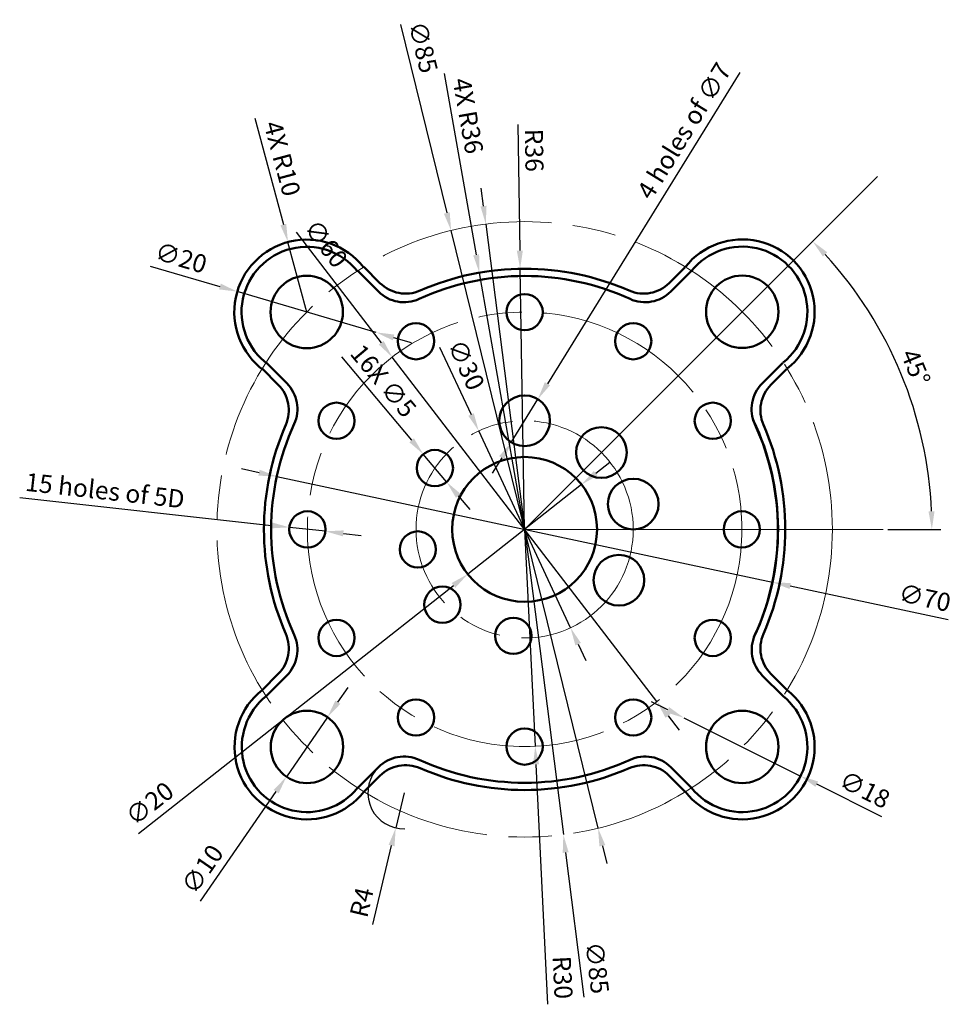
# Model space of a CAD drawing. Units: millimetres. Extents: x 2004 to 2133, y 1449 to 1585.
import ezdxf

# ---------------------------------------------------------------- set-up
doc = ezdxf.new("R2010")
doc.units = ezdxf.units.MM
doc.linetypes.add('ACAD_ISO08W100', pattern=[36, 24, -3, 6, -3])
for name, color, linetype, lineweight in [('M-CNTR', 4, 'ACAD_ISO08W100', 18), ('M-CONS', 8, 'Continuous', 18), ('M-DIMS', 2, 'Continuous', 25), ('M-OUTL', 7, 'Continuous', 50)]:
    doc.layers.add(name, color=color, linetype=linetype, lineweight=lineweight)
doc.styles.get("Standard").update_dxf_attribs({"font": 'arial.ttf'})
doc.dimstyles.new('ISO-25', dxfattribs={"dimtxt": 2.5, "dimasz": 2.5, "dimexe": 1.25, "dimexo": 0.625, "dimtad": 1, "dimdec": 1, "dimdsep": 46, "dimtxsty": 'Standard', "dimcen": 2.5, "dimadec": 0, "dimazin": 0, "dimtfac": 1, "dimtdec": 1, "dimtmove": 0, "dimatfit": 3, "dimfxl": 1, "dimarcsym": 0})

# ---------------------------------------------------------------- blocks, each defined once
blk = doc.blocks.new('*U1')
blk.add_circle((0, 0), 2.5)
blk = doc.blocks.new('*U2')
at = {"layer": 'M-OUTL', "color": 0, "linetype": 'ByBlock', "lineweight": -2, "transparency": 16777216}
blk.add_blockref('*U1', (2074.15, 1544.97), dxfattribs=at)
for p, rotation in [((2059.15, 1540.95), 30), ((2089.15, 1540.95), 330.0000000000001), ((2048.17, 1529.97), 59.99999999999999), ((2100.13, 1529.97), 300), ((2044.15, 1514.97), 90), ((2104.15, 1514.97), 269.9999999999999), ((2048.17, 1499.97), 120), ((2100.13, 1499.97), 240), ((2059.15, 1488.99), 150), ((2089.15, 1488.99), 210), ((2074.15, 1484.97), 180)]:
    blk.add_blockref('*U1', p, dxfattribs=dict(at, rotation=rotation))
blk = doc.blocks.new('*D3')
at = {"layer": 'Defpoints', "color": 0, "lineweight": 100, "transparency": 16777216}
for p in [(2073.53, 1550.97), (2074.15, 1514.97)]:
    blk.add_point(p, dxfattribs=at)
at = {"layer": 'M-DIMS', "color": 0, "lineweight": -2, "transparency": 16777216}
for p, q in [((2073.19, 1570.9), (2073.49, 1553.47)), ((2074.15, 1514.97), (2073.53, 1550.97))]:
    blk.add_line(p, q, dxfattribs=at)
at = {"layer": 'M-DIMS', "color": 0, "lineweight": 100, "transparency": 16777216}
blk.add_solid([(2073.91, 1553.47), (2073.07, 1553.46), (2073.53, 1550.97)], dxfattribs=at)
at = {"layer": 'M-DIMS', "color": 0, "transparency": 16777216, "insert": (2075.15, 1567.32), "char_height": 2.5, "attachment_point": 5, "rotation": 270.9785}
blk.add_mtext('R36', dxfattribs=at)
blk = doc.blocks.new('*D4')
at = {"layer": 'Defpoints', "color": 0, "lineweight": 100, "transparency": 16777216}
for p in [(2034.47, 1547.81), (2053.66, 1542.18)]:
    blk.add_point(p, dxfattribs=at)
at = {"layer": 'M-DIMS', "color": 0, "lineweight": -2, "transparency": 16777216}
for p, q in [((2022.43, 1551.34), (2032.07, 1548.51)), ((2053.66, 1542.18), (2034.47, 1547.81)), ((2056.06, 1541.47), (2058.46, 1540.77))]:
    blk.add_line(p, q, dxfattribs=at)
at = {"layer": 'M-DIMS', "color": 0, "lineweight": 100, "transparency": 16777216}
for points in [[(2032.19, 1548.91), (2031.95, 1548.11), (2034.47, 1547.81)], [(2056.17, 1541.87), (2055.94, 1541.07), (2053.66, 1542.18)]]:
    blk.add_solid(points, dxfattribs=at)
at = {"layer": 'M-DIMS', "color": 0, "transparency": 16777216, "insert": (2026.61, 1552.17), "char_height": 2.5, "attachment_point": 5, "rotation": 343.6386}
blk.add_mtext('∅20', dxfattribs=at)
blk = doc.blocks.new('*D5')
at = {"layer": 'Defpoints', "color": 0, "lineweight": 100, "transparency": 16777216}
for p in [(2039.92, 1522.28), (2108.38, 1507.67)]:
    blk.add_point(p, dxfattribs=at)
at = {"layer": 'M-DIMS', "color": 0, "lineweight": -2, "transparency": 16777216}
for p, q in [((2037.47, 1522.8), (2035.03, 1523.32)), ((2039.92, 1522.28), (2108.38, 1507.67)), ((2132.63, 1502.49), (2110.82, 1507.14))]:
    blk.add_line(p, q, dxfattribs=at)
at = {"layer": 'M-DIMS', "color": 0, "lineweight": 100, "transparency": 16777216}
for points in [[(2037.56, 1523.21), (2037.38, 1522.39), (2039.92, 1522.28)], [(2110.91, 1507.55), (2110.73, 1506.74), (2108.38, 1507.67)]]:
    blk.add_solid(points, dxfattribs=at)
at = {"layer": 'M-DIMS', "color": 0, "transparency": 16777216, "insert": (2129.35, 1505.21), "char_height": 2.5, "attachment_point": 5, "rotation": 347.9527}
blk.add_mtext('∅70', dxfattribs=at)
blk = doc.blocks.new('*D6')
at = {"layer": 'Defpoints', "color": 0, "lineweight": 100, "transparency": 16777216}
for p in [(2096.15, 1488.94), (2112.25, 1480.9)]:
    blk.add_point(p, dxfattribs=at)
at = {"layer": 'M-DIMS', "color": 0, "lineweight": -2, "transparency": 16777216}
for p, q in [((2093.91, 1490.06), (2091.67, 1491.17)), ((2096.15, 1488.94), (2112.25, 1480.9)), ((2123.48, 1475.29), (2114.49, 1479.78))]:
    blk.add_line(p, q, dxfattribs=at)
at = {"layer": 'M-DIMS', "color": 0, "lineweight": 100, "transparency": 16777216}
for points in [[(2094.1, 1490.43), (2093.72, 1489.68), (2096.15, 1488.94)], [(2114.67, 1480.16), (2114.3, 1479.41), (2112.25, 1480.9)]]:
    blk.add_solid(points, dxfattribs=at)
at = {"layer": 'M-DIMS', "color": 0, "transparency": 16777216, "insert": (2120.98, 1478.74), "char_height": 2.5, "attachment_point": 5, "rotation": 333.4694}
blk.add_mtext('∅18', dxfattribs=at)
blk = doc.blocks.new('*D7')
at = {"layer": 'Defpoints', "color": 0, "lineweight": 100, "transparency": 16777216}
for p in [(2068.79, 1557.13), (2079.5, 1472.81)]:
    blk.add_point(p, dxfattribs=at)
at = {"layer": 'M-DIMS', "color": 0, "lineweight": -2, "transparency": 16777216}
for p, q in [((2068.47, 1559.61), (2068.16, 1562.09)), ((2068.79, 1557.13), (2079.5, 1472.81)), ((2082.36, 1450.37), (2079.82, 1470.33))]:
    blk.add_line(p, q, dxfattribs=at)
at = {"layer": 'M-DIMS', "color": 0, "lineweight": 100, "transparency": 16777216}
for points in [[(2068.89, 1559.66), (2068.06, 1559.56), (2068.79, 1557.13)], [(2080.23, 1470.38), (2079.41, 1470.28), (2079.5, 1472.81)]]:
    blk.add_solid(points, dxfattribs=at)
at = {"layer": 'M-DIMS', "color": 0, "transparency": 16777216, "insert": (2083.84, 1454.37), "char_height": 2.5, "attachment_point": 5, "rotation": 277.2438}
blk.add_mtext('∅85', dxfattribs=at)
blk = doc.blocks.new('*D8')
at = {"layer": 'Defpoints', "color": 0, "lineweight": 100, "transparency": 16777216}
for p in [(2074.15, 1514.97), (2075.61, 1485.01)]:
    blk.add_point(p, dxfattribs=at)
at = {"layer": 'M-DIMS', "color": 0, "lineweight": -2, "transparency": 16777216}
for p, q in [((2074.15, 1514.97), (2075.61, 1485.01)), ((2077.35, 1449.38), (2075.73, 1482.51))]:
    blk.add_line(p, q, dxfattribs=at)
at = {"layer": 'M-DIMS', "color": 0, "lineweight": 100, "transparency": 16777216}
blk.add_solid([(2076.15, 1482.53), (2075.32, 1482.49), (2075.61, 1485.01)], dxfattribs=at)
at = {"layer": 'M-DIMS', "color": 0, "transparency": 16777216, "insert": (2079.08, 1453.07), "char_height": 2.5, "attachment_point": 5, "rotation": 272.8002}
blk.add_mtext('R30', dxfattribs=at)
blk = doc.blocks.new('*D9')
at = {"layer": 'Defpoints', "color": 0, "lineweight": 100, "transparency": 16777216}
for p in [(2057.5, 1478.6), (2056.35, 1473.73)]:
    blk.add_point(p, dxfattribs=at)
at = {"layer": 'M-DIMS', "color": 0, "lineweight": -2, "transparency": 16777216}
for p, q in [((2057.5, 1478.6), (2056.35, 1473.73)), ((2053.18, 1460.38), (2055.77, 1471.3))]:
    blk.add_line(p, q, dxfattribs=at)
blk.add_arc((2057.5, 1478.6), 5, 142.1275, 270.9759, dxfattribs=at)
at = {"layer": 'M-DIMS', "color": 0, "lineweight": 100, "transparency": 16777216}
blk.add_solid([(2055.37, 1471.4), (2056.18, 1471.2), (2056.35, 1473.73)], dxfattribs=at)
at = {"layer": 'M-DIMS', "color": 0, "transparency": 16777216, "insert": (2051.96, 1463.38), "char_height": 2.5, "attachment_point": 5, "rotation": 76.652}
blk.add_mtext('R4', dxfattribs=at)
blk = doc.blocks.new('*D10')
at = {"layer": 'Defpoints', "color": 0, "lineweight": 100, "transparency": 16777216}
for p in [(2046.93, 1489.03), (2041.25, 1480.8)]:
    blk.add_point(p, dxfattribs=at)
at = {"layer": 'M-DIMS', "color": 0, "lineweight": -2, "transparency": 16777216}
for p, q in [((2048.35, 1491.09), (2049.77, 1493.15)), ((2046.93, 1489.03), (2041.25, 1480.8)), ((2029.41, 1463.63), (2039.83, 1478.75))]:
    blk.add_line(p, q, dxfattribs=at)
at = {"layer": 'M-DIMS', "color": 0, "lineweight": 100, "transparency": 16777216}
for points in [[(2048.01, 1491.33), (2048.7, 1490.86), (2046.93, 1489.03)], [(2039.49, 1478.98), (2040.18, 1478.51), (2041.25, 1480.8)]]:
    blk.add_solid(points, dxfattribs=at)
at = {"layer": 'M-DIMS', "color": 0, "transparency": 16777216, "insert": (2029.92, 1467.85), "char_height": 2.5, "attachment_point": 5, "rotation": 55.3956}
blk.add_mtext('∅10', dxfattribs=at)
blk = doc.blocks.new('*D11')
at = {"layer": 'Defpoints', "color": 0, "lineweight": 100, "transparency": 16777216}
for p in [(2082, 1521.16), (2066.29, 1508.78)]:
    blk.add_point(p, dxfattribs=at)
at = {"layer": 'M-DIMS', "color": 0, "lineweight": -2, "transparency": 16777216}
for p, q in [((2083.97, 1522.71), (2085.93, 1524.25)), ((2082, 1521.16), (2066.29, 1508.78)), ((2020.81, 1472.96), (2064.33, 1507.24))]:
    blk.add_line(p, q, dxfattribs=at)
at = {"layer": 'M-DIMS', "color": 0, "lineweight": 100, "transparency": 16777216}
for points in [[(2083.71, 1523.03), (2084.22, 1522.38), (2082, 1521.16)], [(2064.07, 1507.56), (2064.58, 1506.91), (2066.29, 1508.78)]]:
    blk.add_solid(points, dxfattribs=at)
at = {"layer": 'M-DIMS', "color": 0, "transparency": 16777216, "insert": (2022.56, 1476.85), "char_height": 2.5, "attachment_point": 5, "rotation": 38.2255}
blk.add_mtext('∅20', dxfattribs=at)
blk = doc.blocks.new('*D12')
at = {"layer": 'Defpoints', "color": 0, "lineweight": 100, "transparency": 16777216}
for p in [(2122.87, 1563.69), (2128.48, 1529.53), (2074.15, 1514.97), (2074.15, 1514.97), (2123.67, 1514.97)]:
    blk.add_point(p, dxfattribs=at)
at = {"layer": 'M-DIMS', "color": 0, "lineweight": -2, "transparency": 16777216}
blk.add_line((2124.29, 1514.97), (2131.64, 1514.97), dxfattribs=at)
blk.add_arc((2074.15, 1514.97), 56.25, 2.5467, 42.4533, dxfattribs=at)
at = {"layer": 'M-DIMS', "color": 0, "lineweight": 100, "transparency": 16777216}
for points in [[(2115.35, 1552.65), (2115.95, 1553.23), (2113.92, 1554.75)], [(2130.76, 1517.48), (2129.92, 1517.46), (2130.39, 1514.97)]]:
    blk.add_solid(points, dxfattribs=at)
at = {"layer": 'M-DIMS', "color": 0, "transparency": 16777216, "insert": (2127.86, 1537.22), "char_height": 2.5, "attachment_point": 5, "rotation": 292.5}
blk.add_mtext('45°', dxfattribs=at)
blk = doc.blocks.new('*D13')
at = {"layer": 'Defpoints', "color": 0, "lineweight": 100, "transparency": 16777216}
for p in [(2041.66, 1515.25), (2046.63, 1514.7)]:
    blk.add_point(p, dxfattribs=at)
at = {"layer": 'M-DIMS', "color": 0, "lineweight": -2, "transparency": 16777216}
for p, q in [((2004.42, 1519.39), (2039.18, 1515.52)), ((2046.63, 1514.7), (2041.66, 1515.25)), ((2049.12, 1514.42), (2051.6, 1514.14))]:
    blk.add_line(p, q, dxfattribs=at)
at = {"layer": 'M-DIMS', "color": 0, "lineweight": 100, "transparency": 16777216}
for points in [[(2039.22, 1515.94), (2039.13, 1515.11), (2041.66, 1515.25)], [(2049.16, 1514.83), (2049.07, 1514), (2046.63, 1514.7)]]:
    blk.add_solid(points, dxfattribs=at)
at = {"layer": 'M-DIMS', "color": 0, "transparency": 16777216, "insert": (2016.17, 1520.01), "char_height": 2.5, "attachment_point": 5, "rotation": 353.6543}
blk.add_mtext('15 holes of 5D', dxfattribs=at)
blk = doc.blocks.new('*D14')
at = {"layer": 'Defpoints', "color": 0, "lineweight": 100, "transparency": 16777216}
for p in [(2075.98, 1532.95), (2072.31, 1526.99)]:
    blk.add_point(p, dxfattribs=at)
at = {"layer": 'M-DIMS', "color": 0, "lineweight": -2, "transparency": 16777216}
for p, q in [((2103.85, 1578.09), (2077.3, 1535.08)), ((2072.31, 1526.99), (2075.98, 1532.95)), ((2070.99, 1524.87), (2069.68, 1522.74))]:
    blk.add_line(p, q, dxfattribs=at)
at = {"layer": 'M-DIMS', "color": 0, "lineweight": 100, "transparency": 16777216}
for points in [[(2076.94, 1535.3), (2077.65, 1534.86), (2075.98, 1532.95)], [(2070.64, 1525.08), (2071.35, 1524.65), (2072.31, 1526.99)]]:
    blk.add_solid(points, dxfattribs=at)
at = {"layer": 'M-DIMS', "color": 0, "transparency": 16777216, "insert": (2096.44, 1569.84), "char_height": 2.5, "attachment_point": 5, "rotation": 58.3122}
blk.add_mtext('4 holes of ∅7', dxfattribs=at)
blk = doc.blocks.new('HOLE-D7')
blk.add_circle((0, 0), 3.5)
blk = doc.blocks.new('HOLE-D5')
blk.add_circle((0, 0), 2.5)
blk = doc.blocks.new('HOLE-D10')
blk.add_circle((0, 0), 5)
blk = doc.blocks.new('*D18')
at = {"layer": 'Defpoints', "color": 0, "lineweight": 100, "transparency": 16777216}
for p in [(2064, 1556.24), (2084.29, 1473.7)]:
    blk.add_point(p, dxfattribs=at)
at = {"layer": 'M-DIMS', "color": 0, "lineweight": -2, "transparency": 16777216}
for p, q in [((2057.01, 1584.68), (2063.4, 1558.67)), ((2084.29, 1473.7), (2064, 1556.24)), ((2084.89, 1471.27), (2085.49, 1468.84))]:
    blk.add_line(p, q, dxfattribs=at)
at = {"layer": 'M-DIMS', "color": 0, "lineweight": 100, "transparency": 16777216}
for points in [[(2063.81, 1558.77), (2063, 1558.57), (2064, 1556.24)], [(2085.29, 1471.37), (2084.48, 1471.17), (2084.29, 1473.7)]]:
    blk.add_solid(points, dxfattribs=at)
at = {"layer": 'M-DIMS', "color": 0, "transparency": 16777216, "insert": (2059.83, 1581.48), "char_height": 2.5, "attachment_point": 5, "rotation": 283.8113}
blk.add_mtext('∅85', dxfattribs=at)
blk = doc.blocks.new('*D19')
at = {"layer": 'Defpoints', "color": 0, "lineweight": 100, "transparency": 16777216}
for p in [(2055.87, 1538.76), (2092.42, 1491.18)]:
    blk.add_point(p, dxfattribs=at)
at = {"layer": 'M-DIMS', "color": 0, "lineweight": -2, "transparency": 16777216}
for p, q in [((2042.61, 1556.03), (2054.35, 1540.74)), ((2092.42, 1491.18), (2055.87, 1538.76)), ((2093.95, 1489.2), (2095.47, 1487.22))]:
    blk.add_line(p, q, dxfattribs=at)
at = {"layer": 'M-DIMS', "color": 0, "lineweight": 100, "transparency": 16777216}
for points in [[(2054.68, 1541), (2054.02, 1540.49), (2055.87, 1538.76)], [(2094.28, 1489.45), (2093.61, 1488.94), (2092.42, 1491.18)]]:
    blk.add_solid(points, dxfattribs=at)
at = {"layer": 'M-DIMS', "color": 0, "transparency": 16777216, "insert": (2046.47, 1554.24), "char_height": 2.5, "attachment_point": 5, "rotation": 307.5327}
blk.add_mtext('∅60', dxfattribs=at)
blk = doc.blocks.new('*D20')
at = {"layer": 'Defpoints', "color": 0, "lineweight": 100, "transparency": 16777216}
for p in [(2067.81, 1528.57), (2080.49, 1501.38)]:
    blk.add_point(p, dxfattribs=at)
at = {"layer": 'M-DIMS', "color": 0, "lineweight": -2, "transparency": 16777216}
for p, q in [((2062.41, 1540.14), (2066.75, 1530.83)), ((2080.49, 1501.38), (2067.81, 1528.57)), ((2081.54, 1499.11), (2082.6, 1496.85))]:
    blk.add_line(p, q, dxfattribs=at)
at = {"layer": 'M-DIMS', "color": 0, "lineweight": 100, "transparency": 16777216}
for points in [[(2067.13, 1531.01), (2066.37, 1530.66), (2067.81, 1528.57)], [(2081.92, 1499.29), (2081.16, 1498.94), (2080.49, 1501.38)]]:
    blk.add_solid(points, dxfattribs=at)
at = {"layer": 'M-DIMS', "color": 0, "transparency": 16777216, "insert": (2065.79, 1537.56), "char_height": 2.5, "attachment_point": 5, "rotation": 295.0007}
blk.add_mtext('∅30', dxfattribs=at)
blk = doc.blocks.new('*D21')
at = {"layer": 'Defpoints', "color": 0, "lineweight": 100, "transparency": 16777216}
for p in [(2060.16, 1525.35), (2063.37, 1521.52)]:
    blk.add_point(p, dxfattribs=at)
at = {"layer": 'M-DIMS', "color": 0, "lineweight": -2, "transparency": 16777216}
for p, q in [((2048.86, 1538.81), (2058.55, 1527.27)), ((2063.37, 1521.52), (2060.16, 1525.35)), ((2064.98, 1519.61), (2066.59, 1517.7))]:
    blk.add_line(p, q, dxfattribs=at)
at = {"layer": 'M-DIMS', "color": 0, "lineweight": 100, "transparency": 16777216}
for points in [[(2058.87, 1527.54), (2058.23, 1527), (2060.16, 1525.35)], [(2065.3, 1519.88), (2064.66, 1519.34), (2063.37, 1521.52)]]:
    blk.add_solid(points, dxfattribs=at)
at = {"layer": 'M-DIMS', "color": 0, "transparency": 16777216, "insert": (2054.41, 1535.27), "char_height": 2.5, "attachment_point": 5, "rotation": 310.0195}
blk.add_mtext('16X ∅5', dxfattribs=at)
blk = doc.blocks.new('*D22')
at = {"layer": 'Defpoints', "color": 0, "lineweight": 100, "transparency": 16777216}
for p in [(2067.9, 1550.42), (2074.15, 1514.97)]:
    blk.add_point(p, dxfattribs=at)
at = {"layer": 'M-DIMS', "color": 0, "lineweight": -2, "transparency": 16777216}
for p, q in [((2063.04, 1577.95), (2067.46, 1552.89)), ((2074.15, 1514.97), (2067.9, 1550.42))]:
    blk.add_line(p, q, dxfattribs=at)
at = {"layer": 'M-DIMS', "color": 0, "lineweight": 100, "transparency": 16777216}
blk.add_solid([(2067.87, 1552.96), (2067.05, 1552.81), (2067.9, 1550.42)], dxfattribs=at)
at = {"layer": 'M-DIMS', "color": 0, "transparency": 16777216, "insert": (2066.02, 1572.03), "char_height": 2.5, "attachment_point": 5, "rotation": 279.9992}
blk.add_mtext('4X R36', dxfattribs=at)
blk = doc.blocks.new('*D23')
at = {"layer": 'Defpoints', "color": 0, "lineweight": 100, "transparency": 16777216}
for p in [(2041.47, 1554.65), (2044.06, 1544.99)]:
    blk.add_point(p, dxfattribs=at)
at = {"layer": 'M-DIMS', "color": 0, "lineweight": -2, "transparency": 16777216}
for p, q in [((2036.9, 1571.74), (2040.83, 1557.07)), ((2044.06, 1544.99), (2041.47, 1554.65))]:
    blk.add_line(p, q, dxfattribs=at)
at = {"layer": 'M-DIMS', "color": 0, "lineweight": 100, "transparency": 16777216}
blk.add_solid([(2041.23, 1557.17), (2040.42, 1556.96), (2041.47, 1554.65)], dxfattribs=at)
at = {"layer": 'M-DIMS', "color": 0, "transparency": 16777216, "insert": (2040.37, 1566.1), "char_height": 2.5, "attachment_point": 5, "rotation": 285.0029}
blk.add_mtext('4X R10', dxfattribs=at)

msp = doc.modelspace()

# ---------------------------------------------------------------- linework, layer by layer
at = {"layer": 'M-CNTR'}
for radius in [42.5, 30, 15]:
    msp.add_circle((2074.15, 1514.97), radius, dxfattribs=at)
at = {"layer": 'M-CONS'}
for q in [(2122.87, 1563.69), (2123.67, 1514.97)]:
    msp.add_line((2074.15, 1514.97), q, dxfattribs=at)
at = {"layer": 'M-OUTL'}
for p, q in [((2051.1, 1550.68), (2053.97, 1547.81)), ((2051.95, 1551.21), (2054.17, 1548.99)), ((2096.28, 1551.15), (2094.12, 1548.99)), ((2097.13, 1550.62), (2094.32, 1547.81)), ((2038.44, 1538.02), (2041.31, 1535.15)), ((2037.9, 1537.17), (2040.13, 1534.94)), ((2109.79, 1537.96), (2106.95, 1535.12)), ((2110.33, 1537.11), (2108.17, 1534.94)), ((2037.9, 1492.77), (2040.13, 1495)), ((2038.44, 1491.92), (2041.31, 1494.8)), ((2109.85, 1491.92), (2106.97, 1494.81)), ((2110.39, 1492.77), (2108.17, 1495)), ((2051.1, 1479.27), (2053.97, 1482.14)), ((2051.95, 1478.73), (2054.17, 1480.95)), ((2096.34, 1478.73), (2094.12, 1480.95)), ((2097.2, 1479.27), (2094.32, 1482.14))]:
    msp.add_line(p, q, dxfattribs=at)
msp.add_circle((2074.15, 1514.97), 10, dxfattribs=at)
for centre, radius, start, end in [((2044.06, 1544.99), 10, 38.3022, 233.6065), ((2104.2, 1545.02), 10, 308.2437, 141.7563), ((2044.06, 1544.99), 9, 38.9805, 233.2797), ((2104.2, 1545.02), 9, 308.922, 141.078), ((2074.15, 1514.97), 36, 66.3597, 113.6402), ((2057.71, 1552.53), 5, 225.0475, 293.6402), ((2074.15, 1514.97), 35, 65.4136, 114.5863), ((2090.59, 1552.53), 5, 246.3597, 314.9525), ((2057.5, 1551.34), 5, 225.0345, 294.5863), ((2090.79, 1551.34), 5, 245.4136, 314.9655), ((2036.59, 1531.41), 5, 336.3598, 44.9525), ((2037.77, 1531.61), 5, 335.4137, 44.9655), ((2110.49, 1531.58), 5, 135.0345, 204.5863), ((2111.71, 1531.41), 5, 135.0475, 203.6403), ((2074.15, 1514.97), 35, 334.8257, 25.54), ((2074.15, 1514.97), 36, 156.3598, 203.6402), ((2074.15, 1514.97), 35, 155.4137, 204.5863), ((2074.12, 1514.94), 35, 335.4801, 24.5863), ((2074.15, 1514.97), 36, 336.3598, 23.6403), ((2074.15, 1514.97), 36, 336.3598, 23.6403), ((2036.59, 1498.53), 5, 315.0475, 23.6402), ((2037.77, 1498.33), 5, 315.0345, 24.5863), ((2110.51, 1498.34), 5, 155.4801, 224.9655), ((2111.71, 1498.53), 5, 156.3598, 224.9525), ((2044.09, 1484.92), 10, 128.2437, 321.7563), ((2044.09, 1484.92), 9, 128.922, 321.078), ((2104.2, 1484.92), 10, 218.2437, 51.7566), ((2104.2, 1484.92), 9, 218.922, 51.078), ((2057.5, 1478.6), 5, 65.4137, 134.9655), ((2057.71, 1477.41), 5, 66.3598, 134.9525), ((2074.15, 1514.97), 35, 245.4137, 294.5863), ((2074.15, 1514.97), 35, 245.4137, 294.5863), ((2090.59, 1477.41), 5, 45.0475, 113.6402), ((2090.79, 1478.6), 5, 45.0345, 114.5863), ((2074.15, 1514.97), 36, 246.3598, 293.6402), ((2074.15, 1514.97), 36, 246.3598, 293.6402)]:
    msp.add_arc(centre, radius, start, end, dxfattribs=at)

# ---------------------------------------------------------------- block references
for name, p in [('HOLE-D10', (2044.06, 1544.99)), ('HOLE-D10', (2104.2, 1545.02)), ('*U2', (0, 0)), ('HOLE-D7', (2074.15, 1529.97)), ('HOLE-D7', (2084.75, 1525.58)), ('HOLE-D5', (2061.76, 1523.44)), ('HOLE-D7', (2089.15, 1518.47)), ('HOLE-D5', (2059.4, 1512.2)), ('HOLE-D7', (2087.17, 1507.95)), ('HOLE-D5', (2062.79, 1504.57)), ('HOLE-D5', (2072.59, 1500.26)), ('HOLE-D10', (2044.09, 1484.92)), ('HOLE-D10', (2104.2, 1484.92))]:
    msp.add_blockref(name, p, dxfattribs=at)

# ---------------------------------------------------------------- dimensions: what is measured, and where the dimension line sits
at = {"layer": 'M-DIMS'}
for p1, p2, override, picture, middle in [((2084.29, 1473.7), (2064, 1556.24), {"dimdec": 0, "dimlfac": 1, "dimrnd": 0, "dimzin": 0, "dimdsep": 46, "dimlunit": 2}, '*D18', (2057.91, 1581.01)), ((2068.79, 1557.13), (2079.5, 1472.81), {"dimclrd": 0, "dimclre": 0, "dimclrt": 0}, '*D7', (2081.88, 1454.12)), ((2092.42, 1491.18), (2055.87, 1538.76), {"dimdec": 0, "dimlfac": 1, "dimrnd": 0, "dimzin": 0, "dimdsep": 46, "dimlunit": 2}, '*D19', (2044.9, 1553.04)), ((2080.49, 1501.38), (2067.81, 1528.57), {"dimdec": 0, "dimlfac": 1, "dimrnd": 0, "dimzin": 0, "dimdsep": 46, "dimlunit": 2}, '*D20', (2064, 1536.72)), ((2082, 1521.16), (2066.29, 1508.78), {"dimclrd": 0, "dimclre": 0, "dimclrt": 0}, '*D11', (2023.78, 1475.3)), ((2039.92, 1522.28), (2108.38, 1507.67), {"dimclrd": 0, "dimclre": 0, "dimclrt": 0}, '*D5', (2128.94, 1503.28)), ((2046.93, 1489.03), (2041.25, 1480.8), {"dimclrd": 0, "dimclre": 0, "dimclrt": 0}, '*D10', (2031.55, 1466.73))]:
    dim = msp.add_diameter_dim_2p(p1=p1, p2=p2, dimstyle='ISO-25', override=override, dxfattribs=at)
    dim.commit()
    dim.dimension.update_dxf_attribs({"geometry": picture, "text_midpoint": middle, "dimtype": 163})
for p1, p2, text, override, picture, middle in [((2072.31, 1526.99), (2075.98, 1532.95), '4 holes of <>', {"dimclrd": 0, "dimclre": 0, "dimclrt": 0}, '*D14', (2098.12, 1568.8)), ((2063.37, 1521.52), (2060.16, 1525.35), '16X <>', {"dimdec": 0, "dimlfac": 1, "dimrnd": 0, "dimzin": 0, "dimdsep": 46, "dimlunit": 2}, '*D21', (2052.9, 1534)), ((2046.63, 1514.7), (2041.66, 1515.25), '15 holes of 5D', {"dimclrd": 0, "dimclre": 0, "dimclrt": 0}, '*D13', (2015.95, 1518.11))]:
    dim = msp.add_diameter_dim_2p(p1=p1, p2=p2, text=text, dimstyle='ISO-25', override=override, dxfattribs=at)
    dim.commit()
    dim.dimension.update_dxf_attribs({"geometry": picture, "text_midpoint": middle, "dimtype": 163})
for center, mpoint, text, override, picture, middle in [((2074.15, 1514.97), (2067.9, 1550.42), '4X <>', {"dimdec": 0, "dimlfac": 1, "dimrnd": 0, "dimzin": 0, "dimdsep": 46, "dimlunit": 2}, '*D22', (2064.14, 1571.7)), ((2057.5, 1478.6), (2056.35, 1473.73), 'R4', {"dimclrd": 0, "dimclre": 0, "dimclrt": 0}, '*D9', (2053.79, 1462.94))]:
    dim = msp.add_radius_dim(center=center, mpoint=mpoint, text=text, dimstyle='ISO-25', override=override, dxfattribs=at)
    dim.commit()
    dim.dimension.update_dxf_attribs({"geometry": picture, "text_midpoint": middle, "dimtype": 164})
dim = msp.add_radius_dim(center=(2044.06, 1544.99), mpoint=(2041.47, 1554.65), text='4X <>', dimstyle='ISO-25', override={"dimdec": 0, "dimlfac": 1, "dimrnd": 0, "dimzin": 0, "dimdsep": 46, "dimlunit": 2}, dxfattribs=at)
dim.commit()
dim.dimension.update_dxf_attribs({"geometry": '*D23', "text_midpoint": (2040.37, 1566.1)})
for mpoint, picture, middle in [((2073.53, 1550.97), '*D3', (2073.25, 1567.29)), ((2075.61, 1485.01), '*D8', (2077.18, 1452.98))]:
    dim = msp.add_radius_dim(center=(2074.15, 1514.97), mpoint=mpoint, dimstyle='ISO-25', override={"dimclrd": 0, "dimclre": 0, "dimclrt": 0}, dxfattribs=at)
    dim.commit()
    dim.dimension.update_dxf_attribs({"geometry": picture, "text_midpoint": middle, "dimtype": 164})
dim = msp.add_angular_dim_2l(base=(2128.48, 1529.53), line1=((2074.15, 1514.97), (2122.87, 1563.69)), line2=((2074.15, 1514.97), (2123.67, 1514.97)), dimstyle='ISO-25', override={"dimclrd": 0, "dimclre": 0, "dimclrt": 0}, dxfattribs=at)
dim.commit()
dim.dimension.update_dxf_attribs({"geometry": '*D12', "text_midpoint": (2127.86, 1537.22)})
for p1, p2, picture, middle in [((2053.66, 1542.18), (2034.47, 1547.81), '*D4', (2026.61, 1552.17)), ((2096.15, 1488.94), (2112.25, 1480.9), '*D6', (2120.98, 1478.74))]:
    dim = msp.add_diameter_dim_2p(p1=p1, p2=p2, dimstyle='ISO-25', override={"dimclrd": 0, "dimclre": 0, "dimclrt": 0}, dxfattribs=at)
    dim.commit()
    dim.dimension.update_dxf_attribs({"geometry": picture, "text_midpoint": middle})

doc.saveas('drawing.dxf')
